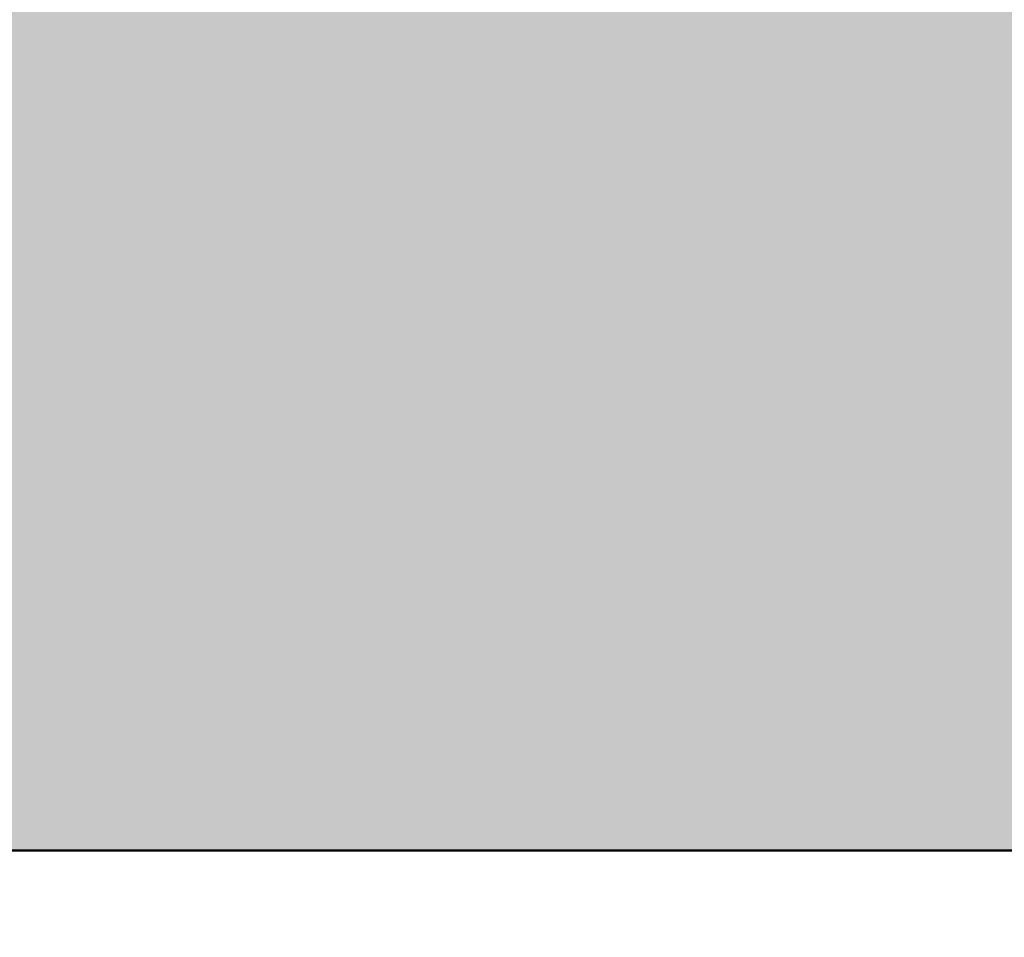
# Model space of a CAD drawing. Units: millimetres. Extents: x 0 to 2267, y 0 to 1823.
# Tile 137 of 256: x 1760 to 1802, y 1074 to 1113. Entities that reach past the tile are written whole.
import ezdxf

# ---------------------------------------------------------------- set-up
doc = ezdxf.new("R2010")
doc.units = ezdxf.units.MM
doc.header["$MEASUREMENT"] = 0
for name, color, linetype, lineweight in [('M-DIMS', 2, 'Continuous', 25), ('M-HATC', 252, 'Continuous', 18), ('M-OUTL', 7, 'Continuous', 50)]:
    doc.layers.add(name, color=color, linetype=linetype, lineweight=lineweight)
doc.styles.get("Standard").update_dxf_attribs({"font": 'arial.ttf'})
doc.dimstyles.get("Standard").update_dxf_attribs({"dimtxt": 7, "dimasz": 4, "dimexe": 0.18, "dimexo": 0.0625, "dimgap": 0.09, "dimtad": 0, "dimdec": 0, "dimzin": 0, "dimdsep": 46, "dimtxsty": 'Standard', "dimcen": 0.09, "dimadec": 0, "dimazin": 0, "dimtfac": 1, "dimtdec": 0, "dimtofl": 0, "dimtmove": 0, "dimatfit": 3, "dimfxl": 1, "dimtolj": 1, "dimtzin": 0, "dimarcsym": 0})

# ---------------------------------------------------------------- blocks, each defined once
blk = doc.blocks.new('*D1')
at = {"layer": 'Defpoints', "color": 0, "transparency": 16777216}
for p in [(1593.429, 1127.417), (1843.429, 1127.417), (1843.429, 955.628)]:
    blk.add_point(p, dxfattribs=at)
at = {"layer": 'M-DIMS', "color": 0, "lineweight": -2, "transparency": 16777216}
for p, q in [((1593.429, 1127.355), (1593.429, 955.448)), ((1843.429, 1127.355), (1843.429, 955.448)), ((1597.429, 955.628), (1710.558, 955.628)), ((1839.429, 955.628), (1726.3, 955.628))]:
    blk.add_line(p, q, dxfattribs=at)
at = {"layer": 'M-DIMS', "color": 0, "transparency": 16777216}
for points in [[(1597.429, 956.294), (1597.429, 954.961), (1593.429, 955.628)], [(1839.429, 956.294), (1839.429, 954.961), (1843.429, 955.628)]]:
    blk.add_solid(points, dxfattribs=at)
at = {"layer": 'M-DIMS', "color": 0, "transparency": 16777216, "insert": (1718.429, 955.628), "char_height": 7, "attachment_point": 5}
blk.add_mtext('\\A1;250', dxfattribs=at)
blk = doc.blocks.new('*D2')
at = {"layer": 'Defpoints', "color": 0, "transparency": 16777216}
for p in [(1505.929, 1077.417), (1930.929, 1077.417), (1930.929, 906.787)]:
    blk.add_point(p, dxfattribs=at)
at = {"layer": 'M-DIMS', "color": 0, "lineweight": -2, "transparency": 16777216}
for p, q in [((1505.929, 1077.355), (1505.929, 906.607)), ((1930.929, 1077.355), (1930.929, 906.607)), ((1509.929, 906.787), (1710.439, 906.787)), ((1926.929, 906.787), (1726.419, 906.787))]:
    blk.add_line(p, q, dxfattribs=at)
at = {"layer": 'M-DIMS', "color": 0, "transparency": 16777216}
for points in [[(1509.929, 907.453), (1509.929, 906.12), (1505.929, 906.787)], [(1926.929, 907.453), (1926.929, 906.12), (1930.929, 906.787)]]:
    blk.add_solid(points, dxfattribs=at)
at = {"layer": 'M-DIMS', "color": 0, "transparency": 16777216, "insert": (1718.429, 906.787), "char_height": 7, "attachment_point": 5}
blk.add_mtext('\\A1;425', dxfattribs=at)

msp = doc.modelspace()

# ---------------------------------------------------------------- hatches: boundary and pattern name
at = {"layer": 'M-HATC'}
h = msp.add_hatch(color=256, dxfattribs=at)
h.dxf.hatch_style = 1
h.paths.add_polyline_path([(2065.771, 1618.062, 0.236068), (2055.771, 1638.062), (1381.087, 1638.062, 0.236068), (1371.087, 1618.062), (1371.087, 1603.062), (2055.771, 1603.062), (2065.771, 1603.062)])
h.paths.add_polyline_path([(2062.772, 1550.296), (2062.772, 1560.296), (1374.086, 1560.296), (1374.086, 1550.296), (1374.086, 1540.296), (1384.086, 1540.296), (1389.086, 1540.296), (2062.772, 1540.296)])
h.paths.add_polyline_path([(1930.929, 1282.766), (1505.929, 1282.766), (1587.628, 1235.597, 0.131652), (1600.128, 1232.247), (1836.73, 1232.247, 0.131652), (1849.23, 1235.597)])
h.paths.add_polyline_path([(1930.929, 1117.417), (1905.929, 1117.417), (1505.929, 1117.417), (1505.929, 1077.417), (1930.929, 1077.417)])

# ---------------------------------------------------------------- linework, layer by layer
at = {"layer": 'M-OUTL'}
msp.add_line((1505.929, 1077.417), (1930.929, 1077.417), dxfattribs=at)

# ---------------------------------------------------------------- dimensions: what is measured, and where the dimension line sits
at = {"layer": 'M-DIMS'}
for base, p1, p2, picture, middle in [((1843.429, 955.628), (1593.429, 1127.417), (1843.429, 1127.417), '*D1', (1718.429, 955.628)), ((1930.929, 906.787), (1505.929, 1077.417), (1930.929, 1077.417), '*D2', (1718.429, 906.787))]:
    dim = msp.add_linear_dim(base=base, p1=p1, p2=p2, dimstyle='Standard', override={"dimclrd": 0, "dimclre": 0, "dimclrt": 0}, dxfattribs=at)
    dim.commit()
    dim.dimension.update_dxf_attribs({"geometry": picture, "text_midpoint": middle})

doc.saveas('drawing.dxf')
